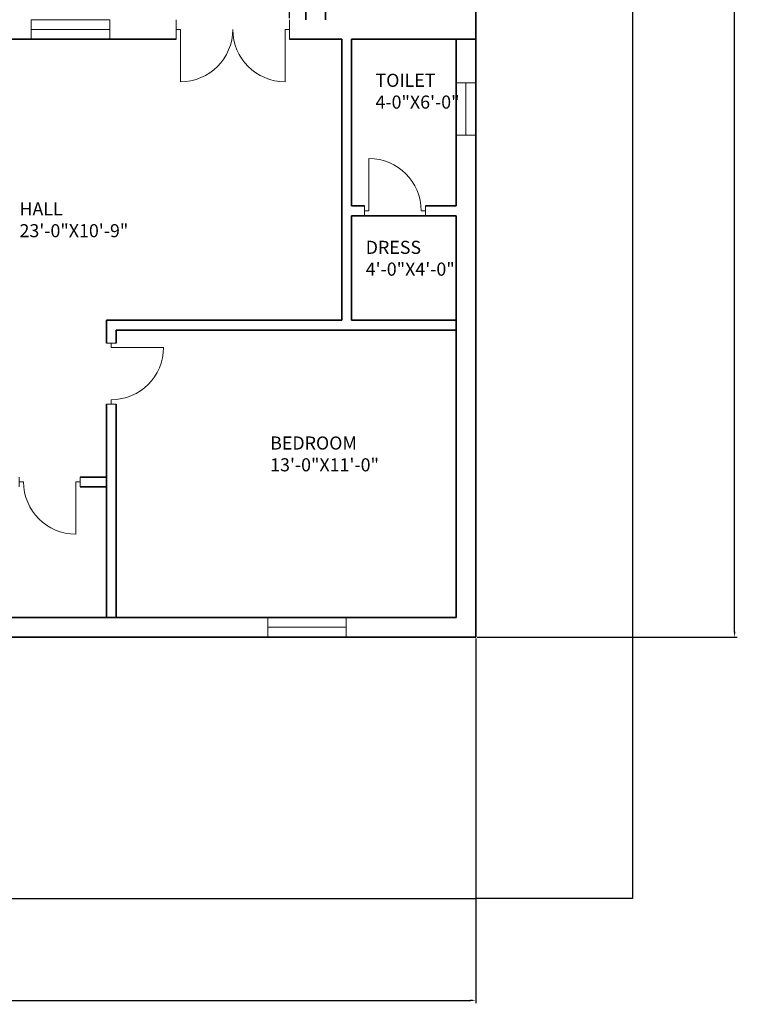
# Model space of a CAD drawing. Units: inches. Extents: x 3257 to 4085, y -12 to 956.
# Tile 3 of 6: x 3755 to 4085, y -12 to 441. Entities that reach past the tile are written whole.
import ezdxf

# ---------------------------------------------------------------- set-up
doc = ezdxf.new("R2010")
doc.units = ezdxf.units.IN
for name, color, linetype, lineweight in [('A-ANNO-DIMS', 2, 'Continuous', 18), ('A-AREA-IDEN', 7, 'Continuous', 18), ('A-DOOR', 3, 'Continuous', 18), ('A-GLAZ', 4, 'Continuous', 18), ('A-WALL', 7, 'Continuous', 35), ('C-PROP', 6, 'Continuous', 25)]:
    doc.layers.add(name, color=color, linetype=linetype, lineweight=lineweight)
doc.styles.get("Standard").update_dxf_attribs({"font": 'arial.ttf'})
doc.dimstyles.new('ISO-25', dxfattribs={"dimtxt": 2.5, "dimasz": 2.5, "dimexe": 1.25, "dimexo": 0.625, "dimtad": 1, "dimdec": 0, "dimlunit": 3, "dimtxsty": 'Standard', "dimcen": 2.5, "dimadec": 0, "dimazin": 0, "dimtfac": 1, "dimtdec": 0, "dimtmove": 0, "dimatfit": 3, "dimfxl": 1, "dimarcsym": 0})

# ---------------------------------------------------------------- blocks, each defined once
blk = doc.blocks.new('DOOR-SGL-24IN')
for p, q in [((2.25, 28), (0, 28)), ((2.25, 26), (2.25, 28)), ((2.25, 28), (4.5, 28)), ((2.25, 0), (2.25, 2)), ((2.25, 2), (26.25, 2)), ((4.5, 0), (0, 0))]:
    blk.add_line(p, q)
blk.add_arc((2.25, 2), 24, 0, 90)
blk = doc.blocks.new('WIN-36IN')
for p, q in [((0, 9), (36, 9)), ((0, 0), (0, 9)), ((36, 9), (36, 0)), ((0, 4.5), (36, 4.5)), ((36, 0), (0, 0))]:
    blk.add_line(p, q)
blk = doc.blocks.new('WIN-24IN')
for p, q in [((0, 9), (24, 9)), ((0, 0), (0, 9)), ((24, 9), (24, 0)), ((0, 4.5), (24, 4.5)), ((24, 0), (0, 0))]:
    blk.add_line(p, q)
blk = doc.blocks.new('DOOR-DBL-2X24IN')
for p, q in [((2, 4.5), (2, 28.5)), ((50, 4.5), (50, 28.5)), ((0, 4.5), (0, 9)), ((52, 9), (52, 0)), ((2, 4.5), (0, 4.5)), ((0, 4.5), (0, 0)), ((52, 4.5), (50, 4.5))]:
    blk.add_line(p, q)
for centre, start, end in [((2, 4.5), 0, 90), ((50, 4.5), 90, 180)]:
    blk.add_arc(centre, 24, start, end)
blk = doc.blocks.new('*D18')
at = {"layer": 'A-ANNO-DIMS', "color": 0, "lineweight": -2, "transparency": 16777216}
for p, q in [((3411.97, 156.38), (3411.97, -11.05)), ((3964.47, 156.38), (3964.47, -11.05)), ((3414.47, -9.8), (3961.97, -9.8))]:
    blk.add_line(p, q, dxfattribs=at)
at = {"layer": 'A-ANNO-DIMS', "color": 0, "transparency": 16777216}
for points in [[(3414.47, -9.38), (3414.47, -10.21), (3411.97, -9.8)], [(3961.97, -9.38), (3961.97, -10.21), (3964.47, -9.8)]]:
    blk.add_solid(points, dxfattribs=at)
at = {"layer": 'Defpoints', "color": 0, "transparency": 16777216}
for p in [(3411.97, 157), (3964.47, 157), (3964.47, -9.8)]:
    blk.add_point(p, dxfattribs=at)
at = {"layer": 'A-ANNO-DIMS', "color": 0, "transparency": 16777216, "insert": (3688.22, -7.88), "char_height": 2.5, "attachment_point": 5}
blk.add_mtext('46\'-0 1/2"', dxfattribs=at)
blk = doc.blocks.new('*D19')
at = {"layer": 'A-ANNO-DIMS', "color": 0, "lineweight": -2, "transparency": 16777216}
for p, q in [((3965.09, 804), (4084.52, 804)), ((4083.27, 159.5), (4083.27, 801.5)), ((3965.09, 157), (4084.52, 157))]:
    blk.add_line(p, q, dxfattribs=at)
at = {"layer": 'A-ANNO-DIMS', "color": 0, "transparency": 16777216}
for points in [[(4082.85, 801.5), (4083.68, 801.5), (4083.27, 804)], [(4082.85, 159.5), (4083.68, 159.5), (4083.27, 157)]]:
    blk.add_solid(points, dxfattribs=at)
at = {"layer": 'Defpoints', "color": 0, "transparency": 16777216}
for p in [(3964.47, 804), (4083.27, 804), (3964.47, 157)]:
    blk.add_point(p, dxfattribs=at)
at = {"layer": 'A-ANNO-DIMS', "color": 0, "transparency": 16777216, "insert": (4081.37, 480.5), "char_height": 2.5, "attachment_point": 5, "rotation": 90}
blk.add_mtext('53\'-11"', dxfattribs=at)
blk = doc.blocks.new('*D25')
at = {"layer": 'A-ANNO-DIMS', "color": 0, "lineweight": -2, "transparency": 16777216}
for p, q in [((3878.97, 441.13), (3878.97, 924.05)), ((3881.47, 922.8), (3883.97, 922.8)), ((3886.47, 441.13), (3886.47, 924.05)), ((3886.47, 922.8), (3902.69, 922.8))]:
    blk.add_line(p, q, dxfattribs=at)
at = {"layer": 'A-ANNO-DIMS', "color": 0, "transparency": 16777216}
for points in [[(3881.47, 923.22), (3881.47, 922.39), (3878.97, 922.8)], [(3883.97, 923.22), (3883.97, 922.39), (3886.47, 922.8)]]:
    blk.add_solid(points, dxfattribs=at)
at = {"layer": 'Defpoints', "color": 0, "transparency": 16777216}
for p in [(3886.47, 922.8), (3878.97, 440.5), (3886.47, 440.5)]:
    blk.add_point(p, dxfattribs=at)
at = {"layer": 'A-ANNO-DIMS', "color": 0, "transparency": 16777216, "insert": (3895.83, 924.72), "char_height": 2.5, "attachment_point": 5}
blk.add_mtext('0\'-7 1/2"', dxfattribs=at)

msp = doc.modelspace()

# ---------------------------------------------------------------- linework, layer by layer
at = {"layer": 'A-WALL'}
for p, q in [((3964.47, 685), (3964.47, 157)), ((3886.47, 524.5), (3886.47, 440.5)), ((3895.47, 524.5), (3895.47, 440.5)), ((3420.97, 431.5), (3826.97, 431.5)), ((3878.97, 431.5), (3902.97, 431.5)), ((3902.97, 431.5), (3902.97, 302.5)), ((3907.47, 431.5), (3907.47, 355)), ((3907.47, 431.5), (3964.47, 431.5)), ((3955.47, 431.5), (3955.47, 355)), ((3907.47, 355), (3913.47, 355)), ((3941.47, 355), (3955.47, 355)), ((3907.47, 350.5), (3955.47, 350.5)), ((3907.47, 350.5), (3907.47, 302.5)), ((3955.47, 350.5), (3955.47, 166)), ((3794.97, 302.5), (3902.97, 302.5)), ((3794.97, 302.5), (3794.97, 292)), ((3907.47, 302.5), (3955.47, 302.5)), ((3799.47, 298), (3799.47, 292)), ((3799.47, 298), (3799.47, 292)), ((3799.47, 298), (3955.47, 298)), ((3794.97, 264), (3794.97, 166)), ((3799.47, 264), (3799.47, 166)), ((3782.97, 230.5), (3794.97, 230.5)), ((3782.97, 226), (3794.97, 226)), ((3420.97, 166), (3955.47, 166)), ((3411.97, 157), (3964.47, 157))]:
    msp.add_line(p, q, dxfattribs=at)
at = {"layer": 'C-PROP'}
for p, q in [((4036.47, 685), (4036.47, 37)), ((3411.97, 37), (3964.47, 37)), ((4036.47, 37), (3964.47, 37))]:
    msp.add_line(p, q, dxfattribs=at)

# ---------------------------------------------------------------- block references
at = {"layer": 'A-DOOR', "extrusion": (0, 0, -1), "zscale": -1}
for name, p, rotation in [('DOOR-DBL-2X24IN', (-3826.97, 440.5), 180), ('DOOR-SGL-24IN', (-3913.47, 350.5), 90.00000000000153), ('DOOR-SGL-24IN', (-3794.97, 292), 180), ('DOOR-SGL-24IN', (-3782.97, 230.5), 269.9999999999985)]:
    msp.add_blockref(name, p, dxfattribs=dict(at, rotation=rotation))
at = {"layer": 'A-GLAZ'}
for name, p, rotation in [('WIN-36IN', (3796.52, 440.5), 180), ('WIN-24IN', (3964.47, 387.44), 89.99999999999729), ('WIN-36IN', (3905.01, 166), 180)]:
    msp.add_blockref(name, p, dxfattribs=dict(at, rotation=rotation))

# ---------------------------------------------------------------- texts
at = {"layer": 'A-AREA-IDEN', "char_height": 6, "attachment_point": 1}
for s, insert in [('TOILET\\P4-0"X6\'-0"', (3918.48, 415.67)), ('HALL\\P23\'-0"X10\'-9"', (3755.11, 356.62)), ('DRESS\\P4\'-0"X4\'-0"', (3913.99, 338.97)), ('BEDROOM\\P13\'-0"X11\'-0"', (3870.14, 249.12))]:
    msp.add_mtext(s, dxfattribs=dict(at, insert=insert))

# ---------------------------------------------------------------- dimensions: what is measured, and where the dimension line sits
at = {"layer": 'A-ANNO-DIMS'}
for base, p1, p2, picture, middle in [((3886.47, 922.8), (3878.97, 440.5), (3886.47, 440.5), '*D25', (3895.83, 924.72)), ((3964.47, -9.8), (3411.97, 157), (3964.47, 157), '*D18', (3688.22, -7.88))]:
    dim = msp.add_linear_dim(base=base, p1=p1, p2=p2, dimstyle='ISO-25', override={"dimdec": 1, "dimlfac": 1, "dimrnd": 0, "dimzin": 1, "dimdsep": 46, "dimlunit": 4, "dimfrac": 2}, dxfattribs=at)
    dim.commit()
    dim.dimension.update_dxf_attribs({"geometry": picture, "text_midpoint": middle})
dim = msp.add_linear_dim(base=(4083.27, 804), p1=(3964.47, 157), p2=(3964.47, 804), angle=90, dimstyle='ISO-25', override={"dimdec": 1, "dimlfac": 1, "dimrnd": 0, "dimzin": 1, "dimdsep": 46, "dimlunit": 4, "dimfrac": 2}, dxfattribs=at)
dim.commit()
dim.dimension.update_dxf_attribs({"geometry": '*D19', "text_midpoint": (4081.37, 480.5)})

doc.saveas('drawing.dxf')
